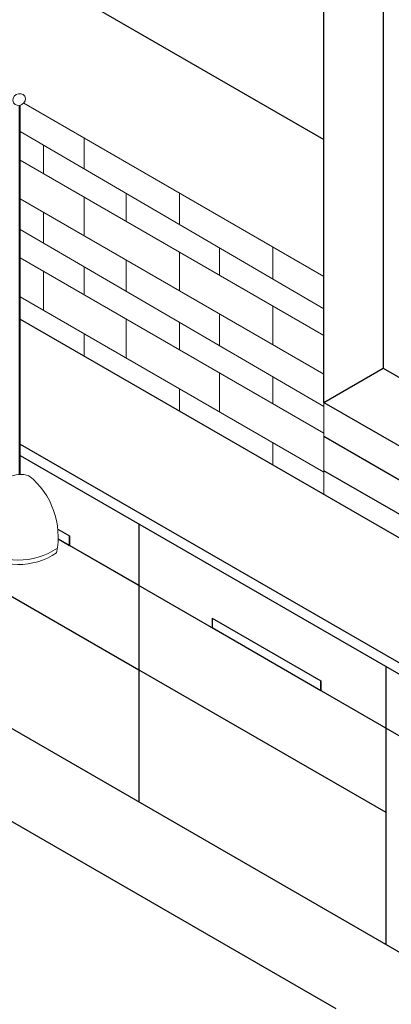
# Model space of a CAD drawing. Units: inches. Extents: x 5770 to 11891, y 3254 to 6808.
# Tile 6 of 15: x 5976 to 6009, y 3403 to 3489. Entities that reach past the tile are written whole.
import ezdxf

# ---------------------------------------------------------------- set-up
doc = ezdxf.new("R2010")
doc.units = ezdxf.units.IN
for name, color, linetype, lineweight in [('A-ANNO-DIMS', 2, 'Continuous', 18), ('A-FURN', 8, 'Continuous', 25), ('A-GLAZ', 4, 'Continuous', 25), ('A-WALL-PATT', 8, 'Continuous', 13), ('E-LITE', 3, 'Continuous', 18)]:
    doc.layers.add(name, color=color, linetype=linetype, lineweight=lineweight)
doc.styles.get("Standard").update_dxf_attribs({"font": 'arial.ttf'})
doc.dimstyles.new('ISO-25', dxfattribs={"dimtxt": 2.5, "dimasz": 2.5, "dimexe": 1.25, "dimexo": 0.625, "dimtad": 1, "dimdec": 0, "dimlunit": 3, "dimtxsty": 'Standard', "dimcen": 2.5, "dimadec": 0, "dimazin": 0, "dimtfac": 1, "dimtdec": 0, "dimtmove": 0, "dimatfit": 3, "dimfxl": 1, "dimarcsym": 0})

# ---------------------------------------------------------------- blocks, each defined once
blk = doc.blocks.new('*D7')
at = {"layer": 'A-ANNO-DIMS', "color": 0, "lineweight": -2, "transparency": 16777216}
for p, q in [((5959.627, 3549.37), (5966.461, 3561.208)), ((5968.001, 3558.875), (6136.876, 3461.375)), ((6132.832, 3449.37), (6139.666, 3461.208))]:
    blk.add_line(p, q, dxfattribs=at)
at = {"layer": 'A-ANNO-DIMS', "color": 0, "transparency": 16777216}
for points in [[(5968.21, 3559.236), (5967.793, 3558.514), (5965.836, 3560.125)], [(6137.085, 3461.736), (6136.668, 3461.014), (6139.041, 3460.125)]]:
    blk.add_solid(points, dxfattribs=at)
at = {"layer": 'Defpoints', "color": 0, "transparency": 16777216}
for p in [(5959.314, 3548.829), (6139.041, 3460.125), (6132.519, 3448.829)]:
    blk.add_point(p, dxfattribs=at)
at = {"layer": 'A-ANNO-DIMS', "color": 0, "transparency": 16777216, "insert": (6061.618, 3507.021), "char_height": 2.5, "attachment_point": 5, "rotation": 330}
blk.add_mtext('16\'-8"', dxfattribs=at)
blk = doc.blocks.new('BULB')
for p, q in [((5936.059, 3465.129), (5936.059, 3432.775)), ((5936.162, 3465.149), (5936.162, 3432.775)), ((5936.059, 3432.775), (5936.162, 3432.775))]:
    blk.add_line(p, q)
for centre, radius, start, end in [((5939.829, 3426.895), 7.337, 129.73045, 187.25106), ((5936.197, 3430.311), 2.466, 73.02955, 115.40364), ((5932.627, 3427.316), 6.859, 348.08023, 51.28845), ((5936.012, 3431.261), 5.994, 234.23536, 304.57537), ((5935.995, 3430.875), 5.994, 234.93114, 303.90063)]:
    blk.add_arc(centre, radius, start, end)
blk.add_ellipse((5936.057, 3465.643), major_axis=(-0.492, -0.284), ratio=0.878374)
blk = doc.blocks.new('CABINET-PULL')
for p, q in [((0, 6.322), (9.524, 0.823)), ((0, 6.322), (0, 5.499)), ((0, 6.322), (0, 5.499)), ((0, 5.499), (9.524, 0)), ((9.524, 0.823), (9.524, 0)), ((9.524, 0), (9.524, 0.823))]:
    blk.add_line(p, q)

msp = doc.modelspace()

# ---------------------------------------------------------------- linework, layer by layer
at = {"layer": 'A-FURN'}
for p, q in [((6002.599, 3455.517), (6002.599, 3497.517)), ((5974.02, 3495.055), (6002.599, 3478.555)), ((5975.971, 3462.811), (6056.394, 3416.379)), ((5975.971, 3451.863), (6059.32, 3403.741)), ((5975.971, 3450.863), (6059.32, 3402.741)), ((6022.299, 3438.144), (6002.599, 3449.517)), ((5964.711, 3444.576), (5986.361, 3432.076)), ((5979.262, 3444.4), (5980.298, 3443.802)), ((5986.361, 3444.864), (5986.361, 3420.496)), ((5979.292, 3443.56), (5980.298, 3442.979)), ((5979.292, 3443.56), (5986.361, 3439.479)), ((5979.292, 3443.56), (6059.32, 3397.356)), ((5980.298, 3443.802), (5980.298, 3442.979)), ((5980.298, 3442.979), (5980.298, 3443.802)), ((5964.711, 3432.996), (6059.32, 3378.374)), ((6008.012, 3432.364), (6008.012, 3407.996)), ((5986.361, 3432.076), (6008.012, 3419.576)), ((5967.262, 3423.368), (6003.635, 3402.368))]:
    msp.add_line(p, q, dxfattribs=at)
at = {"layer": 'A-GLAZ'}
for p, q in [((6007.795, 3494.517), (6007.795, 3458.517)), ((6002.599, 3455.517), (6007.795, 3458.517)), ((6007.795, 3458.517), (6049.365, 3434.517)), ((6002.599, 3455.517), (6015.496, 3448.072)), ((6014.256, 3445.787), (6002.599, 3452.517))]:
    msp.add_line(p, q, dxfattribs=at)
at = {"layer": 'A-WALL-PATT'}
for p, q in [((5976.271, 3481.756), (6002.599, 3466.555)), ((5975.971, 3479.252), (6002.599, 3463.716)), ((5978.008, 3478.063), (5978.008, 3475.575)), ((5981.567, 3478.698), (5981.567, 3475.987)), ((5975.971, 3476.752), (6002.599, 3461.378)), ((5985.265, 3473.829), (5985.265, 3471.386)), ((5989.93, 3473.87), (5989.93, 3471.108)), ((5975.971, 3473.355), (6002.599, 3457.981)), ((5981.567, 3473.521), (5981.567, 3470.124)), ((5978.008, 3472.178), (5978.008, 3469.488)), ((5975.971, 3470.677), (6002.599, 3455.141)), ((5989.93, 3468.692), (5989.93, 3465.296)), ((5993.428, 3469.067), (5993.428, 3466.673)), ((5998.114, 3469.145), (5998.114, 3466.333)), ((5975.971, 3468.177), (6002.599, 3452.803)), ((5985.265, 3467.989), (5985.265, 3465.255)), ((5978.008, 3467.001), (5978.008, 3463.604)), ((5981.567, 3467.412), (5981.567, 3464.946)), ((5975.971, 3464.78), (6002.599, 3449.406)), ((5993.428, 3463.276), (5993.428, 3460.492)), ((5998.114, 3463.967), (5998.114, 3460.57)), ((5985.265, 3462.811), (5985.265, 3459.414)), ((5989.93, 3462.533), (5989.93, 3460.118)), ((5981.567, 3461.549), (5981.567, 3459.58)), ((5993.428, 3458.098), (5993.428, 3454.701)), ((5998.114, 3457.759), (5998.114, 3455.393)), ((5989.93, 3456.721), (5989.93, 3454.752)), ((6002.599, 3455.517), (6002.599, 3447.437)), ((5998.114, 3451.996), (5998.114, 3450.027))]:
    msp.add_line(p, q, dxfattribs=at)

# ---------------------------------------------------------------- block references
at = {"layer": 'A-FURN'}
msp.add_blockref('CABINET-PULL', (5992.792, 3430.267), dxfattribs=at)
at = {"layer": 'E-LITE'}
msp.add_blockref('BULB', (39.809, 16.419), dxfattribs=at)

# ---------------------------------------------------------------- dimensions: what is measured, and where the dimension line sits
at = {"layer": 'A-ANNO-DIMS'}
dim = msp.add_linear_dim(base=(6139.041, 3460.125), p1=(5959.314, 3548.829), p2=(6132.519, 3448.829), angle=330, dimstyle='ISO-25', override={"dimclrd": 0, "dimclre": 0, "dimclrt": 0}, dxfattribs=at)
dim.commit()
dim.dimension.update_dxf_attribs({"geometry": '*D7', "text_midpoint": (6060.667, 3505.374), "dimtype": 161})

doc.saveas('drawing.dxf')
